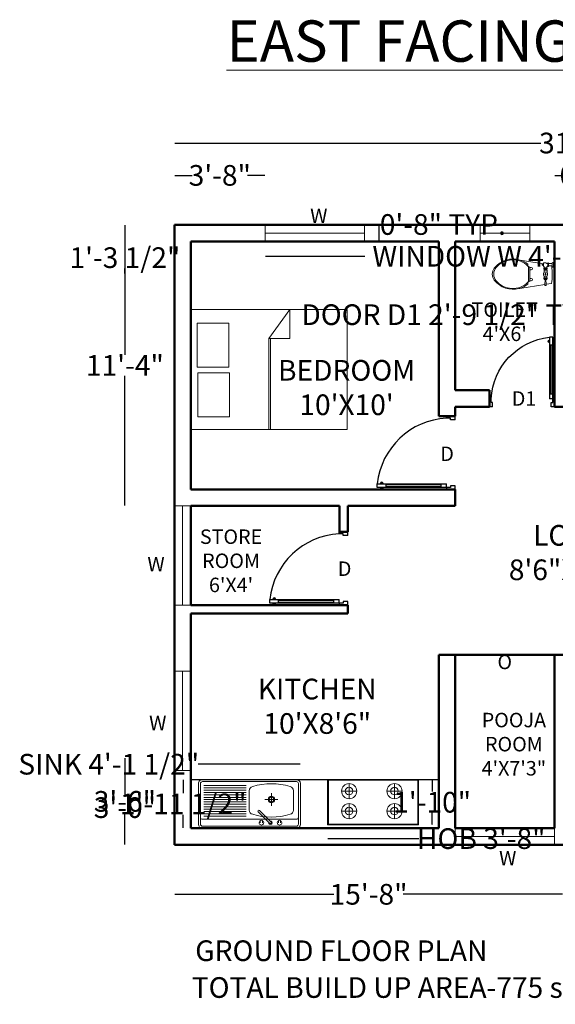
# Model space of a CAD drawing. Units: inches. Extents: x 387 to 883, y 95 to 571.
# Tile 1 of 3: x 387 to 646, y 95 to 571. Entities that reach past the tile are written whole.
import ezdxf

# ---------------------------------------------------------------- set-up
doc = ezdxf.new("R2010")
doc.units = ezdxf.units.IN
doc.header["$MEASUREMENT"] = 0
for name, color, linetype, lineweight in [('A-ANNO-DIMS', 2, 'Continuous', 18), ('A-ANNO-TEXT', 7, 'Continuous', 18), ('A-AREA-IDEN', 7, 'Continuous', 25), ('A-DOOR', 3, 'Continuous', 25), ('A-EQPM', 9, 'Continuous', 18), ('A-FLOR-CASE', 8, 'Continuous', 25), ('A-FLOR-FIXT', 8, 'Continuous', 18), ('A-FURN', 8, 'Continuous', 18), ('A-GLAZ', 4, 'Continuous', 18), ('A-WALL', 7, 'Continuous', 50)]:
    doc.layers.add(name, color=color, linetype=linetype, lineweight=lineweight)
doc.styles.get("Standard").update_dxf_attribs({"font": 'arial.ttf'})
doc.dimstyles.get("Standard").update_dxf_attribs({"dimtxt": 10, "dimasz": 0.18, "dimexe": 0.18, "dimexo": 0.0625, "dimgap": 0.09, "dimtad": 0, "dimtih": 1, "dimtoh": 1, "dimdec": 0, "dimzin": 0, "dimdsep": 46, "dimlunit": 4, "dimtxsty": 'Standard', "dimcen": 0.09, "dimse1": 1, "dimse2": 1, "dimadec": 0, "dimazin": 0, "dimtfac": 1, "dimtdec": 0, "dimtofl": 0, "dimtmove": 0, "dimatfit": 3, "dimfxl": 1, "dimtolj": 1, "dimtzin": 0, "dimarcsym": 0})

# ---------------------------------------------------------------- blocks, each defined once
blk = doc.blocks.new('w')
blk.add_line((755.51, 424.04), (707.51, 424.04))
blk.add_lwpolyline([(707.51, 420.04), (755.51, 420.04), (755.51, 428.04), (707.51, 428.04)], close=True)
blk = doc.blocks.new('w1')
for p, q in [((554.92, 428.04), (554.92, 420.04)), ((554.92, 424.04), (530.92, 424.04))]:
    blk.add_line(p, q)
blk.add_lwpolyline([(554.92, 428.04), (530.92, 428.04), (530.92, 420.04), (554.92, 420.04)])
blk = doc.blocks.new('d1')
for p, q in [((2995.6, 698.54), (2995.6, 699.83)), ((2995.74, 701.33), (2997.52, 701.33)), ((2995.74, 667.71), (2995.74, 701.33)), ((2997.52, 701.33), (2997.52, 667.71)), ((2997.66, 698.54), (2997.66, 699.83)), ((2995.74, 696.72), (2996.1, 696.72)), ((2996.1, 697.09), (2997.16, 697.09)), ((2996.1, 670.28), (2996.1, 697.09)), ((2997.16, 697.09), (2997.16, 670.28)), ((2997.16, 696.72), (2997.52, 696.72)), ((2995.74, 670.55), (2996.1, 670.55)), ((2996.1, 670.28), (2997.16, 670.28)), ((2997.16, 670.55), (2997.52, 670.55)), ((2995.74, 667.71), (2994.8, 667.71)), ((2994.8, 663.45), (2994.8, 667.71)), ((2995.74, 667.71), (2997.52, 667.71)), ((2995.74, 665.76), (2995.74, 667.71)), ((2996.58, 665.76), (2995.74, 665.76)), ((2996.58, 663.45), (2996.58, 665.76)), ((3028.53, 665.76), (3029.37, 665.76)), ((3028.53, 663.45), (3028.53, 665.76)), ((3029.37, 665.76), (3029.37, 667.71)), ((3029.37, 667.71), (3030.3, 667.71)), ((3030.3, 663.45), (3030.3, 667.71)), ((2994.8, 663.45), (2996.58, 663.45)), ((3028.53, 663.45), (3030.3, 663.45))]:
    blk.add_line(p, q)
for centre, radius, start, end in [((2995.6, 699.19), 0.641, 90, 270), ((2993.79, 665.9), 35.62, 2.9057, 83.9884), ((2997.66, 699.19), 0.641, 270, 90)]:
    blk.add_arc(centre, radius, start, end)
blk = doc.blocks.new('BED')
for p, q in [((1734.1, 2886.7), (1849.5, 2886.7)), ((1734.1, 2884.7), (1849.5, 2884.7)), ((1849.5, 2886.7), (1886.1, 2860.2)), ((1886.1, 2860.2), (1849.5, 2886.7)), ((1849.5, 2886.7), (1849.5, 2860.2)), ((1849.5, 2860.2), (1886.1, 2860.2))]:
    blk.add_line(p, q)
for points in [[(1734.1, 2787.7), (1886.1, 2787.7), (1886.1, 2985.7), (1734.1, 2985.7)], [(1750, 2936.8), (1805.9, 2936.8), (1805.9, 2977), (1750, 2977)], [(1813.2, 2937.8), (1869.1, 2937.8), (1869.1, 2977.9), (1813.2, 2977.9)]]:
    blk.add_lwpolyline(points, close=True)
blk = doc.blocks.new('s')
for p, q in [((942.3, 155.1), (942.3, 95.1)), ((942.3, 155.1), (1062.3, 155.1)), ((943.3, 154.1), (943.3, 96.1)), ((943.3, 154.1), (1061.3, 154.1)), ((970.7, 129.8), (970.7, 149.8)), ((1030.6, 149.8), (1030.6, 129.8)), ((1061.3, 154.1), (1061.3, 96.1)), ((1062.3, 155.1), (1062.3, 95.1)), ((960.7, 139.8), (980.7, 139.8)), ((970.7, 139.8), (970.7, 129.8)), ((1020.6, 139.8), (1040.6, 139.8)), ((970.7, 103.4), (970.7, 123.4)), ((1030.6, 103.4), (1030.6, 123.4)), ((980.7, 113.4), (960.7, 113.4)), ((1040.6, 113.4), (1020.6, 113.4)), ((1062.3, 95.1), (942.3, 95.1)), ((1061.3, 96.1), (943.3, 96.1))]:
    blk.add_line(p, q)
for centre, radius in [((970.7, 139.8), 10), ((970.7, 139.8), 5), ((1030.6, 139.8), 10), ((1030.6, 139.8), 5), ((970.7, 113.4), 10), ((970.7, 113.4), 5), ((1030.6, 113.4), 10), ((1030.6, 113.4), 5)]:
    blk.add_circle(centre, radius)
blk = doc.blocks.new('A$C24281843')
for p, q in [((0, 0.742), (0, 0.067)), ((1.637, 0.66), (0.056, 0.66)), ((0.134, 0.66), (0.056, 0.66)), ((1.626, 0.81), (0.067, 0.81)), ((0.067, 0.776), (1.626, 0.776)), ((0.328, 0.681), (0.328, 0.718)), ((0.366, 0.681), (0.366, 0.718)), ((0.487, 0.708), (0.681, 0.514)), ((0.701, 0.534), (0.507, 0.728)), ((0.628, 0.681), (0.628, 0.718)), ((0.666, 0.681), (0.666, 0.718)), ((1.693, 0.067), (1.693, 0.742)), ((0.115, 0.508), (0.115, 0.186)), ((0.85, 0.186), (0.85, 0.508)), ((0.902, 0.607), (1.607, 0.607)), ((0.902, 0.568), (1.607, 0.568)), ((0.902, 0.529), (1.607, 0.529)), ((0.375, 0.332), (0.59, 0.332)), ((0.482, 0.439), (0.482, 0.224)), ((0.902, 0.49), (1.607, 0.49)), ((0.902, 0.451), (1.607, 0.451)), ((0.902, 0.412), (1.607, 0.412)), ((0.902, 0.373), (1.607, 0.373)), ((0.902, 0.334), (1.607, 0.334)), ((0.902, 0.296), (1.607, 0.296)), ((0.902, 0.257), (1.607, 0.257)), ((0.902, 0.218), (1.607, 0.218)), ((0.902, 0.179), (1.607, 0.179)), ((0.067, 0.034), (1.626, 0.034)), ((0.902, 0.14), (1.607, 0.14)), ((0.902, 0.101), (1.607, 0.101)), ((1.626, 0), (0.067, 0))]:
    blk.add_line(p, q)
for points in [[(0.034, 0.742), (0.034, 0.067)], [(1.66, 0.067), (1.66, 0.742)]]:
    blk.add_lwpolyline(points)
for points in [[(0.172, 0.576, -0.154641), (0.792, 0.576)], [(0.172, 0.117, 0.154641), (0.792, 0.117, -0.022148)]]:
    blk.add_lwpolyline(points, format="xyb")
for radius in [0.0538, 0.0403]:
    blk.add_circle((0.482, 0.332), radius)
for centre, radius, start, end in [((0.067, 0.742), 0.0675, 90, 180), ((0.067, 0.742), 0.0338, 90, 180), ((0.056, 0.637), 0.0225, 90, 180), ((0.347, 0.718), 0.0375, 300, 240), ((0.347, 0.706), 0.0318, 233.9153, 306.0847), ((0.497, 0.718), 0.0281, 345, 285), ((0.497, 0.718), 0.0141, 45, 225), ((0.647, 0.718), 0.0375, 300, 240), ((0.647, 0.706), 0.0318, 233.9153, 306.0847), ((1.626, 0.742), 0.0675, 0, 90), ((1.626, 0.742), 0.0338, 0, 90), ((1.637, 0.637), 0.0225, 0, 90), ((0.184, 0.508), 0.07, 100.6708, 179.5694), ((0.691, 0.524), 0.0141, 225, 45), ((0.78, 0.508), 0.07, 0.4306, 79.3292), ((0.184, 0.186), 0.07, 180.4306, 259.3292), ((0.78, 0.186), 0.07, 280.6708, 359.5694), ((0.067, 0.067), 0.0675, 180, 270), ((0.067, 0.067), 0.0338, 180, 270), ((1.626, 0.067), 0.0675, 270, 0), ((1.626, 0.067), 0.0338, 270, 0)]:
    blk.add_arc(centre, radius, start, end)
blk = doc.blocks.new('TOILETY')
for p, q in [((2296.18, 1053.04), (2296.18, 1053.32)), ((2296.61, 1052.51), (2296.98, 1052.51)), ((2296.98, 1052.51), (2297.74, 1052.51)), ((2297.74, 1052.61), (2297.74, 1052.53)), ((2297.74, 1052.53), (2297.74, 1052.51)), ((2297.74, 1052.51), (2297.74, 1050.24)), ((2297.74, 1050.24), (2297.74, 1050.17)), ((2303.23, 1052.05), (2303.23, 1050.7)), ((2307.26, 1052.61), (2307.26, 1052.53)), ((2307.26, 1052.53), (2307.26, 1052.51)), ((2307.26, 1052.51), (2307.26, 1050.24)), ((2307.26, 1050.24), (2307.26, 1050.17)), ((2296.53, 1036.19), (2297.18, 1037.38)), ((2297.18, 1037.38), (2297.18, 1038.67)), ((2299.5, 1037.38), (2297.18, 1037.38)), ((2299.5, 1038.67), (2299.5, 1037.38)), ((2303.22, 1037.38), (2299.5, 1037.38)), ((2303.22, 1037.38), (2306.94, 1037.38)), ((2306.94, 1038.67), (2306.94, 1037.38)), ((2306.94, 1037.38), (2309.26, 1037.38)), ((2309.26, 1037.38), (2309.26, 1038.67)), ((2309.9, 1036.19), (2309.26, 1037.38))]:
    blk.add_line(p, q)
for points in [[(2293.85, 1057.29), (2293.28, 1057.29, -0.293225), (2292.64, 1058.42), (2294.98, 1058.42), (2297.17, 1058.42, -0.293225), (2296.54, 1057.29), (2295.97, 1057.29)], [(2290.73, 1028.75), (2293.96, 1049.64, -0.075157)], [(2293.85, 1054.1), (2293.63, 1054.1, 0.913215), (2293.63, 1053.32)], [(2294.98, 1057.29), (2293.85, 1057.29, -0.293225)], [(2294.91, 1054.1), (2293.85, 1054.1, 0.913215)], [(2294.91, 1054.1), (2295.97, 1054.1, -0.913215)], [(2294.98, 1057.29), (2295.97, 1057.29, 0.335115)], [(2295.97, 1056.9, -0.066772), (2311.57, 1056.74, -11.173493)], [(2295.97, 1054.1), (2296.18, 1054.1, -0.913215), (2296.18, 1053.32), (2296.11, 1053.32)], [(2297.78, 1052.66, 0.071269), (2297.81, 1052.53, 0.085783), (2297.9, 1052.35, 0.10607), (2298.04, 1052.23, 0.126822), (2298.2, 1052.19, 0.126822), (2298.36, 1052.23, 0.10607), (2298.5, 1052.35, 0.085783), (2298.59, 1052.53, 0.071269), (2298.62, 1052.66, 0.075445)], [(2297.78, 1050.12, -0.056795), (2297.81, 1050.29, -0.085783), (2297.9, 1050.46, -0.10607), (2298.04, 1050.59, -0.126822), (2298.2, 1050.63, -0.126822), (2298.36, 1050.59, -0.10607), (2298.5, 1050.46, -0.085783), (2298.59, 1050.29, -0.056795), (2298.62, 1050.12, -0.075445)], [(2298.66, 1052.58, 0.236068), (2298.84, 1052.47), (2299.76, 1052.47, 0.868488)], [(2298.66, 1050.17, -0.236068), (2298.84, 1050.28), (2299.76, 1050.28, -0.868488)], [(2306.34, 1052.58, -0.236068), (2306.17, 1052.47), (2304.79, 1052.47, -0.947474)], [(2306.34, 1050.17, 0.236068), (2306.17, 1050.28), (2304.79, 1050.28, 0.947474)], [(2307.23, 1052.66, -0.071269), (2307.19, 1052.53, -0.085783), (2307.1, 1052.35, -0.10607), (2306.96, 1052.23, -0.126822), (2306.8, 1052.19, -0.126822), (2306.65, 1052.23, -0.10607), (2306.5, 1052.35, -0.085783), (2306.41, 1052.53, -0.071269), (2306.38, 1052.66, -0.075445)], [(2307.23, 1050.12, 0.056795), (2307.19, 1050.29, 0.085783), (2307.1, 1050.46, 0.10607), (2306.96, 1050.59, 0.126822), (2306.8, 1050.63, 0.126822), (2306.65, 1050.59, 0.10607), (2306.5, 1050.46, 0.085783), (2306.41, 1050.29, 0.056795), (2306.38, 1050.12, 0.075445)], [(2307.26, 1052.51, 0.414214), (2307.4, 1052.44), (2307.9, 1052.47, -0.274044), (2308.04, 1052.4), (2308.04, 1051.9)], [(2307.26, 1050.24, -0.414214), (2307.4, 1050.31), (2307.9, 1050.28, 0.274044), (2308.04, 1050.35), (2308.04, 1050.84)], [(2308.04, 1051.9, 0.386607), (2308.25, 1051.76), (2312.2, 1051.98, -0.016038)], [(2308.04, 1050.84, -0.386607), (2308.25, 1050.98), (2312.4, 1050.75, 0.016063)], [(2312.2, 1051.98), (2311.57, 1056.74, 0.064477)], [(2312.2, 1051.98), (2312.68, 1052.01, -0.016603), (2312.71, 1052.01, -1.33807)], [(2312.4, 1050.75), (2312.68, 1050.74, 0.016603), (2312.71, 1050.74, 1.33807)], [(2315.84, 1028.5), (2312.4, 1050.75, 0.07524)], [(2312.71, 1052.01, -0.398884), (2313.25, 1051.55), (2313.25, 1051.37)], [(2312.71, 1050.74, 0.398884), (2313.25, 1051.2), (2313.25, 1051.37)], [(2296.03, 1035.7, 0.434217), (2297.18, 1007.59, 0.182634), (2303.22, 1005.38, 2.693815)], [(2294.42, 1035.7, 0.094048), (2290.73, 1028.75, 0.16845)], [(2296.03, 1035.7), (2294.42, 1035.7, 0.416606)], [(2296.53, 1036.19, 0.008985), (2296.03, 1035.7, 0.182634)], [(2303.22, 1036.19), (2296.53, 1036.19, 0.008985)], [(2303.22, 1036.19), (2309.9, 1036.19, -0.444938)], [(2310.4, 1035.7, -0.434217), (2309.26, 1007.59, -0.182634), (2303.22, 1005.38, -2.693815)], [(2309.9, 1036.19, -0.008985), (2310.4, 1035.7, -0.182634)], [(2310.4, 1035.7), (2312.01, 1035.7, -0.416606)], [(2312.01, 1035.7, -0.105447), (2315.97, 1027.83, -0.16845)], [(2290.73, 1028.75, 0.310397), (2297.82, 1005.91, 0.16845), (2303.22, 1004.04, 2.883082)], [(2315.97, 1027.83, -0.298065), (2308.61, 1005.91, -0.16845), (2303.22, 1004.04, -2.883082)], [(2315.97, 1027.83, 0.006132), (2315.84, 1028.5, 0.069947)]]:
    blk.add_lwpolyline(points, format="xyb")
for points in [[(2293.63, 1053.32), (2293.63, 1052.54), (2293.28, 1051.76), (2293.28, 1049.78)], [(2293.96, 1049.64), (2293.35, 1049.64), (2293.28, 1049.78)], [(2296.18, 1053.32), (2293.63, 1053.32)], [(2293.85, 1054.1), (2293.85, 1057.29)], [(2294.24, 1049.64), (2293.96, 1049.64)], [(2294.17, 1049.46), (2294.24, 1049.46)], [(2294.34, 1048.89), (2294.17, 1048.89), (2294.17, 1049.46)], [(2294.17, 1049.46), (2294.45, 1049.38), (2294.81, 1049.46), (2295.16, 1049.38), (2295.44, 1049.46)], [(2294.17, 1048.89), (2294.45, 1048.96), (2294.81, 1048.89), (2295.16, 1048.96), (2295.44, 1048.89)], [(2294.24, 1049.46), (2294.24, 1049.64)], [(2295.37, 1049.64), (2294.24, 1049.64)], [(2294.24, 1049.46), (2295.37, 1049.46)], [(2294.34, 1048.89), (2294.34, 1048.51), (2294.58, 1048.51)], [(2295.26, 1048.89), (2294.34, 1048.89)], [(2294.45, 1048.96), (2294.45, 1049.38)], [(2294.58, 1048.51), (2295.26, 1048.51), (2295.26, 1048.89)], [(2295.16, 1048.96), (2295.16, 1049.38)], [(2295.37, 1049.46), (2295.44, 1049.46), (2295.44, 1048.89), (2295.26, 1048.89)], [(2296.32, 1049.78), (2296.25, 1049.64), (2295.37, 1049.64)], [(2295.37, 1049.46), (2295.37, 1049.64)], [(2295.97, 1056.9), (2295.97, 1057.29)], [(2295.97, 1054.1), (2295.97, 1056.9)], [(2296.33, 1049.78), (2296.56, 1050.24)], [(2296.56, 1050.24), (2297.74, 1050.24)], [(2298.66, 1050.17), (2298.66, 1052.61)], [(2299.76, 1052.51), (2299.76, 1052.72), (2301.87, 1052.72)], [(2299.76, 1052.51), (2299.76, 1050.28)], [(2299.76, 1050.28), (2299.76, 1050.06), (2301.84, 1050.06)], [(2306.34, 1050.17), (2306.34, 1052.61)], [(2308.04, 1051.9), (2308.04, 1051.37)], [(2308.04, 1050.84), (2308.04, 1051.37)]]:
    blk.add_lwpolyline(points)
for points in [[(2294.91, 1053.32, 0.06206), (2295.16, 1053.35, 0.075298), (2295.36, 1053.43, 0.107049), (2295.5, 1053.57, 0.150029), (2295.55, 1053.71, 0.150029), (2295.5, 1053.85, 0.107049), (2295.36, 1053.99, 0.075298), (2295.16, 1054.07, 0.06206), (2294.91, 1054.1, 0.06206), (2294.65, 1054.07, 0.075298), (2294.46, 1053.99, 0.107049), (2294.31, 1053.85, 0.150029), (2294.27, 1053.71, 0.150029), (2294.31, 1053.57, 0.107049), (2294.46, 1053.43, 0.075298), (2294.65, 1053.35, 0.06206)], [(2298.63, 1051.37, -0.075445), (2298.59, 1051.15, -0.085783), (2298.5, 1050.97, -0.10607), (2298.36, 1050.85, -0.126822), (2298.2, 1050.81, -0.126822), (2298.04, 1050.85, -0.10607), (2297.9, 1050.97, -0.085783), (2297.81, 1051.15, -0.075445), (2297.78, 1051.37, -0.075445), (2297.81, 1051.6, -0.085783), (2297.9, 1051.77, -0.10607), (2298.04, 1051.9, -0.126822), (2298.2, 1051.94, -0.126822), (2298.36, 1051.9, -0.10607), (2298.5, 1051.77, -0.085783), (2298.59, 1051.6, -0.075445)], [(2306.38, 1051.37, 0.075445), (2306.41, 1051.15, 0.085783), (2306.5, 1050.97, 0.10607), (2306.65, 1050.85, 0.126822), (2306.8, 1050.81, 0.126822), (2306.96, 1050.85, 0.10607), (2307.1, 1050.97, 0.085783), (2307.19, 1051.15, 0.075445), (2307.23, 1051.37, 0.075445), (2307.19, 1051.6, 0.085783), (2307.1, 1051.77, 0.10607), (2306.96, 1051.9, 0.126822), (2306.8, 1051.94, 0.126822), (2306.65, 1051.9, 0.10607), (2306.5, 1051.77, 0.085783), (2306.41, 1051.6, 0.075445)]]:
    blk.add_lwpolyline(points, format="xyb", close=True)
blk.add_lwpolyline([(2303.23, 1052.05), (2302.65, 1051.71), (2302.65, 1051.04), (2303.23, 1050.7), (2303.81, 1051.04), (2303.81, 1051.71)], close=True)
blk.add_circle((2303.23, 1051.37), 1.91)
for centre, radius, start, end in [((2293.74, 1053.71), 0.391, 275.19443, 84.80557), ((2296.08, 1053.71), 0.391, 95.19443, 264.80557), ((2296.71, 1053.02), 0.527, 178.46083, 258.85878), ((2298.2, 1052.31), 0.551, 33.39849, 146.60151), ((2298.2, 1050.47), 0.551, 213.39849, 326.60151), ((2306.8, 1052.31), 0.551, 33.39849, 146.60151), ((2306.8, 1050.47), 0.551, 213.39849, 326.60151), ((2298.34, 1038.67), 1.16, 0, 180), ((2308.1, 1038.67), 1.16, 0, 180)]:
    blk.add_arc(centre, radius, start, end)
blk = doc.blocks.new('*D11')
at = {"layer": 'A-ANNO-DIMS', "color": 0, "lineweight": -2, "transparency": 16777216}
for p, q in [((462.03, 511.61), (639.28, 511.61)), ((833.67, 511.61), (656.42, 511.61))]:
    blk.add_line(p, q, dxfattribs=at)
at = {"layer": 'A-ANNO-DIMS', "color": 0, "transparency": 16777216}
for points in [[(462.03, 511.64), (462.03, 511.58), (461.85, 511.61)], [(833.67, 511.64), (833.67, 511.58), (833.85, 511.61)]]:
    blk.add_solid(points, dxfattribs=at)
at = {"layer": 'Defpoints', "color": 0, "transparency": 16777216}
for p in [(461.85, 511.61), (461.85, 472), (833.85, 472)]:
    blk.add_point(p, dxfattribs=at)
at = {"layer": 'A-ANNO-DIMS', "color": 0, "transparency": 16777216, "insert": (647.85, 511.61), "char_height": 10, "attachment_point": 5}
blk.add_mtext("\\A1;31'", dxfattribs=at)
blk = doc.blocks.new('*D13')
at = {"layer": 'A-ANNO-DIMS', "color": 0, "lineweight": -2, "transparency": 16777216}
for p, q in [((506.03, 456.8), (553.67, 456.8)), ((553.85, 456.8), (554.03, 456.8))]:
    blk.add_line(p, q, dxfattribs=at)
at = {"layer": 'A-ANNO-DIMS', "color": 0, "transparency": 16777216}
for points in [[(506.03, 456.83), (506.03, 456.77), (505.85, 456.8)], [(553.67, 456.83), (553.67, 456.77), (553.85, 456.8)]]:
    blk.add_solid(points, dxfattribs=at)
at = {"layer": 'Defpoints', "color": 0, "transparency": 16777216}
for p in [(505.85, 464), (553.85, 464), (553.85, 456.8)]:
    blk.add_point(p, dxfattribs=at)
at = {"layer": 'A-ANNO-DIMS', "color": 0, "transparency": 16777216, "insert": (625.93, 456.8), "char_height": 10, "attachment_point": 5}
blk.add_mtext('\\A1;WINDOW W 4\'-0" TYP.', dxfattribs=at)
blk = doc.blocks.new('*D14')
at = {"layer": 'A-ANNO-DIMS', "color": 0, "lineweight": -2, "transparency": 16777216}
for p, q in [((561.05, 472), (561.05, 472.18)), ((561.05, 472.18), (561.23, 472.18)), ((561.05, 464.18), (561.05, 471.82))]:
    blk.add_line(p, q, dxfattribs=at)
at = {"layer": 'A-ANNO-DIMS', "color": 0, "transparency": 16777216}
for points in [[(561.02, 471.82), (561.08, 471.82), (561.05, 472)], [(561.02, 464.18), (561.08, 464.18), (561.05, 464)]]:
    blk.add_solid(points, dxfattribs=at)
at = {"layer": 'Defpoints', "color": 0, "transparency": 16777216}
for p in [(553.85, 472), (561.05, 472), (553.85, 464)]:
    blk.add_point(p, dxfattribs=at)
at = {"layer": 'A-ANNO-DIMS', "color": 0, "transparency": 16777216, "insert": (591.8, 472.18), "char_height": 10, "attachment_point": 5}
blk.add_mtext('\\A1;0\'-8" TYP.', dxfattribs=at)
blk = doc.blocks.new('*D17')
at = {"layer": 'A-ANNO-DIMS', "color": 0, "lineweight": -2, "transparency": 16777216}
for p, q in [((672.24, 428.54), (672.06, 428.54)), ((705.67, 428.54), (672.42, 428.54))]:
    blk.add_line(p, q, dxfattribs=at)
at = {"layer": 'A-ANNO-DIMS', "color": 0, "transparency": 16777216}
for points in [[(672.42, 428.57), (672.42, 428.51), (672.24, 428.54)], [(705.67, 428.57), (705.67, 428.51), (705.85, 428.54)]]:
    blk.add_solid(points, dxfattribs=at)
at = {"layer": 'Defpoints', "color": 0, "transparency": 16777216}
for p in [(672.24, 428.54), (672.24, 423.5), (705.85, 423.5)]:
    blk.add_point(p, dxfattribs=at)
at = {"layer": 'A-ANNO-DIMS', "color": 0, "transparency": 16777216, "insert": (596.32, 428.54), "char_height": 10, "attachment_point": 5}
blk.add_mtext('\\A1;DOOR D1 2\'-9 1/2" TYP.', dxfattribs=at)
blk = doc.blocks.new('*D25')
at = {"layer": 'A-ANNO-DIMS', "color": 0, "lineweight": -2, "transparency": 16777216}
for p, q in [((536.21, 175), (579.85, 175)), ((580.03, 175), (580.21, 175))]:
    blk.add_line(p, q, dxfattribs=at)
at = {"layer": 'A-ANNO-DIMS', "color": 0, "transparency": 16777216}
for points in [[(536.21, 175.03), (536.21, 174.97), (536.03, 175)], [(579.85, 175.03), (579.85, 174.97), (580.03, 175)]]:
    blk.add_solid(points, dxfattribs=at)
at = {"layer": 'Defpoints', "color": 0, "transparency": 16777216}
for p in [(536.03, 181.6), (580.03, 181.6), (580.03, 175)]:
    blk.add_point(p, dxfattribs=at)
at = {"layer": 'A-ANNO-DIMS', "color": 0, "transparency": 16777216, "insert": (610.39, 175), "char_height": 10, "attachment_point": 5}
blk.add_mtext('\\A1;HOB 3\'-8"', dxfattribs=at)
blk = doc.blocks.new('*D26')
at = {"layer": 'A-ANNO-DIMS', "color": 0, "lineweight": -2, "transparency": 16777216}
for p, q in [((586.63, 203.42), (586.63, 197.79)), ((586.63, 181.78), (586.63, 187.4))]:
    blk.add_line(p, q, dxfattribs=at)
at = {"layer": 'A-ANNO-DIMS', "color": 0, "transparency": 16777216}
for points in [[(586.6, 203.42), (586.66, 203.42), (586.63, 203.6)], [(586.6, 181.78), (586.66, 181.78), (586.63, 181.6)]]:
    blk.add_solid(points, dxfattribs=at)
at = {"layer": 'Defpoints', "color": 0, "transparency": 16777216}
for p in [(580.03, 203.6), (586.63, 203.6), (580.03, 181.6)]:
    blk.add_point(p, dxfattribs=at)
at = {"layer": 'A-ANNO-DIMS', "color": 0, "transparency": 16777216, "insert": (586.63, 192.6), "char_height": 10, "attachment_point": 5}
blk.add_mtext('\\A1;1\'-10"', dxfattribs=at)
blk = doc.blocks.new('*D27')
at = {"layer": 'A-ANNO-DIMS', "color": 0, "lineweight": -2, "transparency": 16777216}
for p, q in [((473.53, 211), (473.35, 211)), ((522.68, 211), (473.71, 211))]:
    blk.add_line(p, q, dxfattribs=at)
at = {"layer": 'A-ANNO-DIMS', "color": 0, "transparency": 16777216}
for points in [[(473.71, 211.03), (473.71, 210.97), (473.53, 211)], [(522.68, 211.03), (522.68, 210.97), (522.86, 211)]]:
    blk.add_solid(points, dxfattribs=at)
at = {"layer": 'Defpoints', "color": 0, "transparency": 16777216}
for p in [(473.53, 211), (473.53, 203.6), (522.86, 203.6)]:
    blk.add_point(p, dxfattribs=at)
at = {"layer": 'A-ANNO-DIMS', "color": 0, "transparency": 16777216, "insert": (430.09, 211), "char_height": 10, "attachment_point": 5}
blk.add_mtext('\\A1;SINK 4\'-1 1/2"', dxfattribs=at)
blk = doc.blocks.new('*D28')
at = {"layer": 'A-ANNO-DIMS', "color": 0, "lineweight": -2, "transparency": 16777216}
for p, q in [((466.13, 203.42), (466.13, 197.06)), ((466.13, 180.18), (466.13, 186.54))]:
    blk.add_line(p, q, dxfattribs=at)
at = {"layer": 'A-ANNO-DIMS', "color": 0, "transparency": 16777216}
for points in [[(466.1, 203.42), (466.16, 203.42), (466.13, 203.6)], [(466.1, 180.18), (466.16, 180.18), (466.13, 180)]]:
    blk.add_solid(points, dxfattribs=at)
at = {"layer": 'Defpoints', "color": 0, "transparency": 16777216}
for p in [(473.53, 203.6), (466.13, 180), (473.53, 180)]:
    blk.add_point(p, dxfattribs=at)
at = {"layer": 'A-ANNO-DIMS', "color": 0, "transparency": 16777216, "insert": (466.13, 191.8), "char_height": 10, "attachment_point": 5}
blk.add_mtext('\\A1;1\'-11 1/2"', dxfattribs=at)
blk = doc.blocks.new('*D33')
at = {"layer": 'A-ANNO-DIMS', "color": 0, "lineweight": -2, "transparency": 16777216}
for p, q in [((462.03, 495.95), (470.47, 495.95)), ((505.67, 495.95), (497.23, 495.95))]:
    blk.add_line(p, q, dxfattribs=at)
at = {"layer": 'A-ANNO-DIMS', "color": 0, "transparency": 16777216}
for points in [[(462.03, 495.98), (462.03, 495.92), (461.85, 495.95)], [(505.67, 495.98), (505.67, 495.92), (505.85, 495.95)]]:
    blk.add_solid(points, dxfattribs=at)
at = {"layer": 'Defpoints', "color": 0, "transparency": 16777216}
for p in [(505.85, 495.95), (461.85, 472), (505.85, 472)]:
    blk.add_point(p, dxfattribs=at)
at = {"layer": 'A-ANNO-DIMS', "color": 0, "transparency": 16777216, "insert": (483.85, 495.95), "char_height": 10, "attachment_point": 5}
blk.add_mtext('\\A1;3\'-8"', dxfattribs=at)
blk = doc.blocks.new('*D35')
at = {"layer": 'A-ANNO-DIMS', "color": 0, "lineweight": -2, "transparency": 16777216}
for p, q in [((437.9, 471.82), (437.9, 409.11)), ((437.9, 336.18), (437.9, 398.89))]:
    blk.add_line(p, q, dxfattribs=at)
at = {"layer": 'A-ANNO-DIMS', "color": 0, "transparency": 16777216}
for points in [[(437.87, 471.82), (437.93, 471.82), (437.9, 472)], [(437.87, 336.18), (437.93, 336.18), (437.9, 336)]]:
    blk.add_solid(points, dxfattribs=at)
at = {"layer": 'Defpoints', "color": 0, "transparency": 16777216}
for p in [(437.9, 472), (461.85, 472), (461.85, 336)]:
    blk.add_point(p, dxfattribs=at)
at = {"layer": 'A-ANNO-DIMS', "color": 0, "transparency": 16777216, "insert": (437.9, 404), "char_height": 10, "attachment_point": 5}
blk.add_mtext('\\A1;11\'-4"', dxfattribs=at)
blk = doc.blocks.new('*D36')
at = {"layer": 'A-ANNO-DIMS', "color": 0, "lineweight": -2, "transparency": 16777216}
for p, q in [((437.9, 207.82), (437.9, 195.2)), ((437.9, 172.18), (437.9, 184.8))]:
    blk.add_line(p, q, dxfattribs=at)
at = {"layer": 'A-ANNO-DIMS', "color": 0, "transparency": 16777216}
for points in [[(437.87, 207.82), (437.93, 207.82), (437.9, 208)], [(437.87, 172.18), (437.93, 172.18), (437.9, 172)]]:
    blk.add_solid(points, dxfattribs=at)
at = {"layer": 'Defpoints', "color": 0, "transparency": 16777216}
for p in [(437.9, 208), (461.85, 208), (461.85, 172)]:
    blk.add_point(p, dxfattribs=at)
at = {"layer": 'A-ANNO-DIMS', "color": 0, "transparency": 16777216, "insert": (437.9, 190), "char_height": 10, "attachment_point": 5}
blk.add_mtext('\\A1;3\'-0"', dxfattribs=at)
blk = doc.blocks.new('*D38')
at = {"layer": 'A-ANNO-DIMS', "color": 0, "lineweight": -2, "transparency": 16777216}
for p, q in [((462.03, 148.05), (539.06, 148.05)), ((649.67, 148.05), (572.65, 148.05))]:
    blk.add_line(p, q, dxfattribs=at)
at = {"layer": 'A-ANNO-DIMS', "color": 0, "transparency": 16777216}
for points in [[(462.03, 148.08), (462.03, 148.02), (461.85, 148.05)], [(649.67, 148.08), (649.67, 148.02), (649.85, 148.05)]]:
    blk.add_solid(points, dxfattribs=at)
at = {"layer": 'Defpoints', "color": 0, "transparency": 16777216}
for p in [(461.85, 172), (649.85, 172), (649.85, 148.05)]:
    blk.add_point(p, dxfattribs=at)
at = {"layer": 'A-ANNO-DIMS', "color": 0, "transparency": 16777216, "insert": (555.85, 148.05), "char_height": 10, "attachment_point": 5}
blk.add_mtext('\\A1;15\'-8"', dxfattribs=at)
blk = doc.blocks.new('*D41')
at = {"layer": 'A-ANNO-DIMS', "color": 0, "lineweight": -2, "transparency": 16777216}
for p, q in [((646.03, 495.95), (649.67, 495.95)), ((649.85, 495.95), (650.03, 495.95))]:
    blk.add_line(p, q, dxfattribs=at)
at = {"layer": 'A-ANNO-DIMS', "color": 0, "transparency": 16777216}
for points in [[(646.03, 495.98), (646.03, 495.92), (645.85, 495.95)], [(649.67, 495.98), (649.67, 495.92), (649.85, 495.95)]]:
    blk.add_solid(points, dxfattribs=at)
at = {"layer": 'Defpoints', "color": 0, "transparency": 16777216}
for p in [(649.85, 495.95), (645.85, 464), (649.85, 464)]:
    blk.add_point(p, dxfattribs=at)
at = {"layer": 'A-ANNO-DIMS', "color": 0, "transparency": 16777216, "insert": (663.41, 495.95), "char_height": 10, "attachment_point": 5}
blk.add_mtext('\\A1;0\'-4"', dxfattribs=at)
blk = doc.blocks.new('*D43')
at = {"layer": 'A-ANNO-DIMS', "color": 0, "lineweight": -2, "transparency": 16777216}
for p, q in [((437.9, 213.86), (437.9, 198.22)), ((437.9, 172.18), (437.9, 187.82))]:
    blk.add_line(p, q, dxfattribs=at)
at = {"layer": 'A-ANNO-DIMS', "color": 0, "transparency": 16777216}
for points in [[(437.87, 213.86), (437.93, 213.86), (437.9, 214.04)], [(437.87, 172.18), (437.93, 172.18), (437.9, 172)]]:
    blk.add_solid(points, dxfattribs=at)
at = {"layer": 'Defpoints', "color": 0, "transparency": 16777216}
for p in [(437.9, 214.04), (650.89, 214.04), (649.85, 172)]:
    blk.add_point(p, dxfattribs=at)
at = {"layer": 'A-ANNO-DIMS', "color": 0, "transparency": 16777216, "insert": (437.9, 193.02), "char_height": 10, "attachment_point": 5}
blk.add_mtext('\\A1;3\'-6"', dxfattribs=at)
blk = doc.blocks.new('*D44')
at = {"layer": 'A-ANNO-DIMS', "color": 0, "lineweight": -2, "transparency": 16777216}
for p, q in [((437.9, 463.82), (437.9, 461.41)), ((437.9, 448.47), (437.9, 450.88))]:
    blk.add_line(p, q, dxfattribs=at)
at = {"layer": 'A-ANNO-DIMS', "color": 0, "transparency": 16777216}
for points in [[(437.87, 463.82), (437.93, 463.82), (437.9, 464)], [(437.87, 448.47), (437.93, 448.47), (437.9, 448.29)]]:
    blk.add_solid(points, dxfattribs=at)
at = {"layer": 'Defpoints', "color": 0, "transparency": 16777216}
for p in [(649.85, 464), (437.9, 448.29), (668.2, 448.29)]:
    blk.add_point(p, dxfattribs=at)
at = {"layer": 'A-ANNO-DIMS', "color": 0, "transparency": 16777216, "insert": (437.9, 456.14), "char_height": 10, "attachment_point": 5}
blk.add_mtext('\\A1;1\'-3 1/2"', dxfattribs=at)

msp = doc.modelspace()

# ---------------------------------------------------------------- linework, layer by layer
at = {"layer": 'A-FLOR-CASE'}
msp.add_line((469.85, 203.6), (589.85, 203.6), dxfattribs=at)
at = {"layer": 'A-WALL'}
for p, q in [((461.85, 172), (461.85, 472)), ((461.85, 472), (833.85, 472)), ((469.85, 464), (589.85, 464)), ((469.85, 344), (469.85, 464)), ((589.85, 379.4), (589.85, 464)), ((597.85, 464), (645.85, 464)), ((597.85, 392), (597.85, 464)), ((645.85, 384), (645.85, 464)), ((597.85, 392), (614.45, 392)), ((614.45, 384), (614.45, 392)), ((597.85, 384), (614.45, 384)), ((597.85, 379.4), (597.85, 384)), ((645.85, 384), (697.85, 384)), ((589.85, 379.4), (597.85, 379.4)), ((469.85, 344), (597.85, 344)), ((597.85, 336), (597.85, 344)), ((469.85, 336), (541.85, 336)), ((469.85, 288), (469.85, 336)), ((541.85, 323.4), (541.85, 336)), ((545.85, 323.4), (545.85, 336)), ((545.85, 336), (597.85, 336)), ((541.85, 323.4), (545.85, 323.4)), ((469.85, 288), (545.85, 288)), ((545.85, 284), (545.85, 288)), ((469.85, 180), (469.85, 284)), ((469.85, 284), (545.85, 284)), ((589.85, 180), (589.85, 264)), ((589.85, 264), (649.85, 264)), ((597.85, 180), (597.85, 264)), ((645.85, 180), (645.85, 264)), ((469.85, 180), (589.85, 180)), ((597.85, 180), (645.85, 180)), ((461.85, 172), (649.85, 172))]:
    msp.add_line(p, q, dxfattribs=at)

# ---------------------------------------------------------------- block references
at = {"layer": 'A-DOOR', "xscale": -0.8873243955715187, "yscale": 0.8873243955715187, "zscale": 0.8873243955715187}
msp.add_blockref('d1', (3303.21, -204.7), dxfattribs=at)
at = {"layer": 'A-DOOR', "xscale": 0.9971830985915492, "yscale": 0.9971830985915492, "zscale": 0.9971830985915492, "rotation": 90.00000000000003}
for p in [(1259.43, -2642.37), (1207.43, -2698.37)]:
    msp.add_blockref('d1', p, dxfattribs=at)
at = {"layer": 'A-EQPM', "xscale": 0.3666666666666667, "yscale": 0.3666666666666667, "zscale": 0.3666666666666667}
msp.add_blockref('s', (190.51, 146.73), dxfattribs=at)
at = {"layer": 'A-FLOR-FIXT'}
for name, p, xscale, yscale, zscale, rotation in [('TOILETY', (68.3, 1703.87), 0.5452019050314921, 0.5452019050314921, 0.5452019050314921, 270), ('A$C24281843', (522.86, 203.6), 29.13580246913581, 29.13580246913581, 29.13580246913581, 180)]:
    msp.add_blockref(name, p, dxfattribs=dict(at, xscale=xscale, yscale=yscale, zscale=zscale, rotation=rotation))
at = {"layer": 'A-FURN', "xscale": 0.381578947368421, "yscale": 0.381578947368421, "zscale": 0.381578947368421, "rotation": 89.99999999999999}
msp.add_blockref('BED', (1609.15, -288.71), dxfattribs=at)
at = {"layer": 'A-GLAZ'}
for name, p in [('w', (-201.66, 43.96)), ('w1', (78.93, 43.96)), ('w', (-109.66, -248.04))]:
    msp.add_blockref(name, p, dxfattribs=at)
at = {"layer": 'A-GLAZ', "rotation": 90}
for p in [(889.89, -419.51), (889.89, -499.51)]:
    msp.add_blockref('w', p, dxfattribs=at)

# ---------------------------------------------------------------- texts
at = {"layer": 'A-ANNO-TEXT', "attachment_point": 1}
for s, width, insert, char_height in [('{\\fArial|b1|i0|c0|p34;\\LEAST FACING HOUSE\\l }', 366.1947, (487.14, 570.93), 20), ('\\pxqc;W', 47.8337, (507.85, 479.89), 7), ('\\pxqc;D1', 47.8337, (607.22, 391.48), 7), ('\\pxqc;D', 47.8337, (569.97, 364.72), 7), ('\\pxqc;W', 47.8337, (429.06, 311.35), 7), ('\\pxqc;D', 47.8337, (520.35, 309.11), 7), ('\\pxqc;O', 47.8337, (597.85, 264), 7), ('\\pxqc;W', 47.8337, (429.9, 234.46), 7), ('\\pxqc;W', 47.8337, (599.3, 169.09), 7), ('{\\fArial|b1|i0|c0|p34;GROUND FLOOR PLAN}', 260.4105, (471.93, 125.75), 10), ('TOTAL BUILD UP AREA-775 sq ft', 214.2919, (470.27, 107.95), 10)]:
    msp.add_mtext_dynamic_manual_height_columns(s, width=width, gutter_width=1, heights=[0], dxfattribs=dict(at, insert=insert, char_height=char_height))
at = {"layer": 'A-AREA-IDEN', "attachment_point": 1}
for s, width, insert, char_height in [("\\pxqc;TOILET\\P4'X6'", 47.8337, (597.85, 434.45), 7), ("\\pxqc;BEDROOM\\P10'X10'", 47.8337, (521.28, 406.61), 10), ("\\pxqc;STORE ROOM\\P6'X4'", 54.8823, (461.85, 324.61), 7), ('\\pxqc;LOBBY\\P8\'6"X10\'3"', 47.8337, (632.93, 326.75), 10), ('\\pxqc;KITCHEN\\P10\'X8\'6"', 47.8337, (507.1, 252.38), 10), ('\\pxqc;POOJA ROOM\\P4\'X7\'3"', 47.8337, (602.29, 235.88), 7)]:
    msp.add_mtext_dynamic_manual_height_columns(s, width=width, gutter_width=1, heights=[0], dxfattribs=dict(at, insert=insert, char_height=char_height))

# ---------------------------------------------------------------- dimensions: what is measured, and where the dimension line sits
at = {"layer": 'A-ANNO-DIMS'}
dim = msp.add_aligned_dim(p1=(833.85, 472), p2=(461.85, 472), distance=-39.61, dimstyle='Standard', override={"dimclrd": 0, "dimclre": 0, "dimclrt": 0}, dxfattribs=at)
dim.commit()
dim.dimension.update_dxf_attribs({"geometry": '*D11', "text_midpoint": (647.85, 511.61)})
for base, p1, p2, picture, middle in [((505.85, 495.95), (461.85, 472), (505.85, 472), '*D33', (483.85, 495.95)), ((649.85, 495.95), (645.85, 464), (649.85, 464), '*D41', (663.41, 495.95)), ((649.85, 148.05), (461.85, 172), (649.85, 172), '*D38', (555.85, 148.05))]:
    dim = msp.add_linear_dim(base=base, p1=p1, p2=p2, dimstyle='Standard', override={"dimdec": 1, "dimlfac": 1, "dimrnd": 0, "dimzin": 1, "dimdsep": 46, "dimlunit": 4, "dimfrac": 2}, dxfattribs=at)
    dim.commit()
    dim.dimension.update_dxf_attribs({"geometry": picture, "text_midpoint": middle})
for base, p1, p2, text, picture, middle in [((553.85, 456.8), (505.85, 464), (553.85, 464), 'WINDOW W <> TYP.', '*D13', (625.93, 456.8)), ((580.03, 175), (536.03, 181.6), (580.03, 181.6), 'HOB <>', '*D25', (610.39, 175))]:
    dim = msp.add_linear_dim(base=base, p1=p1, p2=p2, text=text, dimstyle='Standard', override={"dimdec": 1, "dimlfac": 1, "dimrnd": 0, "dimzin": 1, "dimdsep": 46, "dimlunit": 4, "dimfrac": 2}, dxfattribs=at)
    dim.commit()
    dim.dimension.update_dxf_attribs({"geometry": picture, "text_midpoint": middle})
for base, p1, p2, angle, text, picture, middle in [((561.05, 472), (553.85, 464), (553.85, 472), 90, '<> TYP.', '*D14', (591.8, 472.18)), ((672.24, 428.54), (705.85, 423.5), (672.24, 423.5), 180, 'DOOR D1 <> TYP.', '*D17', (596.32, 428.54)), ((473.53, 211), (522.86, 203.6), (473.53, 203.6), 180, 'SINK <>', '*D27', (430.09, 211))]:
    dim = msp.add_linear_dim(base=base, p1=p1, p2=p2, angle=angle, text=text, dimstyle='Standard', override={"dimdec": 1, "dimlfac": 1, "dimrnd": 0, "dimzin": 1, "dimdsep": 46, "dimlunit": 4, "dimfrac": 2}, dxfattribs=at)
    dim.commit()
    dim.dimension.update_dxf_attribs({"geometry": picture, "text_midpoint": middle})
for base, p1, p2, angle, picture, middle in [((437.9, 472), (461.85, 336), (461.85, 472), 90, '*D35', (437.9, 404)), ((437.9, 448.29), (649.85, 464), (668.2, 448.29), 90, '*D44', (437.9, 456.14)), ((437.9, 214.04), (649.85, 172), (650.89, 214.04), 90, '*D43', (437.9, 193.02)), ((437.9, 208), (461.85, 172), (461.85, 208), 90, '*D36', (437.9, 190)), ((466.13, 180), (473.53, 203.6), (473.53, 180), 270, '*D28', (466.13, 191.8)), ((586.63, 203.6), (580.03, 181.6), (580.03, 203.6), 90, '*D26', (586.63, 192.6))]:
    dim = msp.add_linear_dim(base=base, p1=p1, p2=p2, angle=angle, dimstyle='Standard', override={"dimdec": 1, "dimlfac": 1, "dimrnd": 0, "dimzin": 1, "dimdsep": 46, "dimlunit": 4, "dimfrac": 2}, dxfattribs=at)
    dim.commit()
    dim.dimension.update_dxf_attribs({"geometry": picture, "text_midpoint": middle})

doc.saveas('drawing.dxf')
